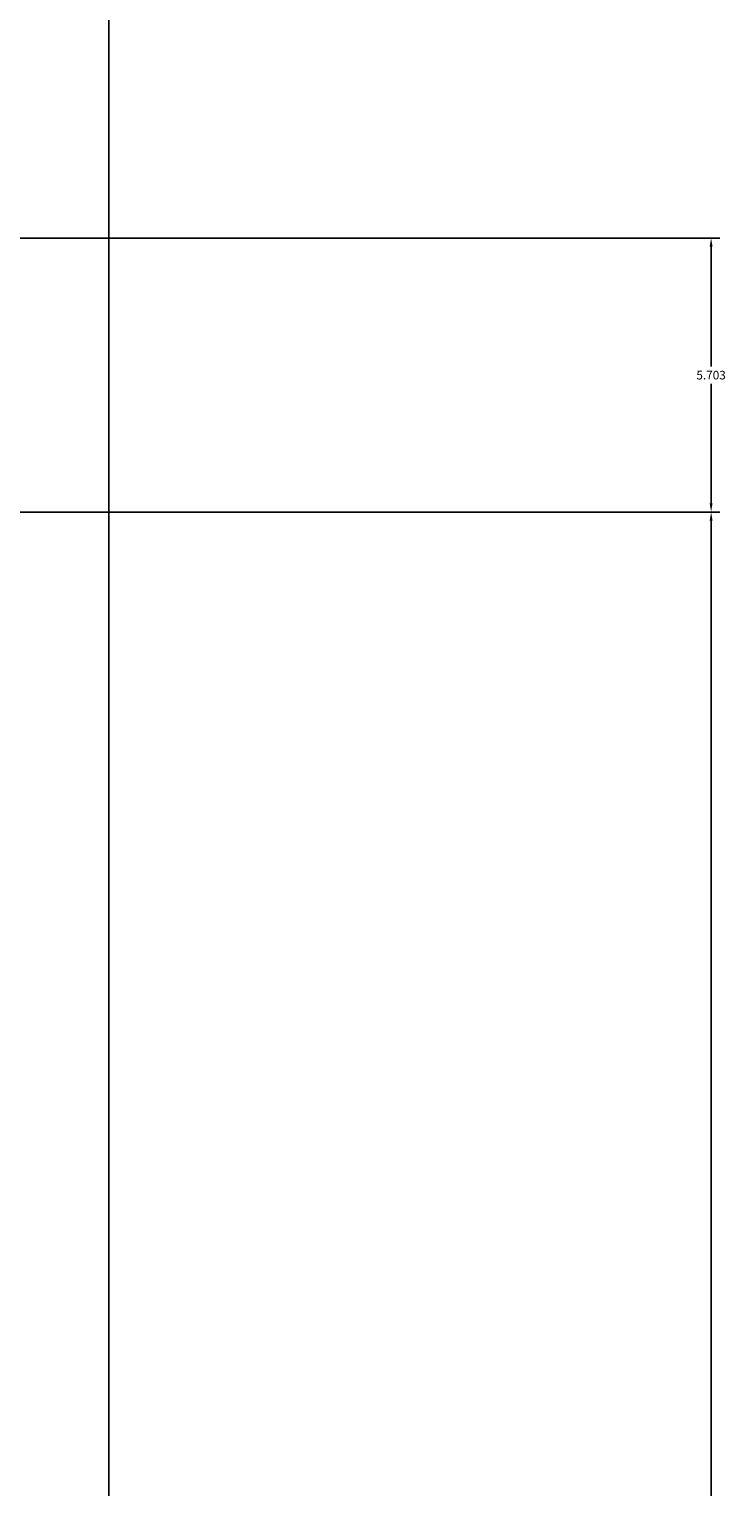
# Model space of a CAD drawing. Units: inches. Extents: x 2812 to 3051, y 1398 to 1659.
# Tile 42 of 65: x 3037 to 3051, y 1468 to 1498. Entities that reach past the tile are written whole.
import ezdxf

# ---------------------------------------------------------------- set-up
doc = ezdxf.new("R2010")
doc.units = ezdxf.units.IN
doc.layers.add('A-ANNO-DIMS', color=2, linetype='Continuous', lineweight=18)
doc.styles.get("Standard").update_dxf_attribs({"font": 'arial.ttf'})
doc.dimstyles.get("Standard").update_dxf_attribs({"dimtxt": 0.18, "dimasz": 0.18, "dimexe": 0.18, "dimexo": 0.0625, "dimgap": 0.09, "dimtad": 0, "dimtih": 1, "dimtoh": 1, "dimdec": 4, "dimzin": 0, "dimdsep": 46, "dimtxsty": 'Standard', "dimcen": 0.09, "dimadec": 0, "dimazin": 0, "dimtfac": 1, "dimtdec": 4, "dimtofl": 0, "dimtmove": 0, "dimatfit": 3, "dimfxl": 1, "dimtolj": 1, "dimtzin": 0, "dimarcsym": 0})

# ---------------------------------------------------------------- blocks, each defined once
blk = doc.blocks.new('*D34')
at = {"layer": 'A-ANNO-DIMS', "color": 0, "lineweight": -2, "transparency": 16777216}
for p, q in [((3038.462, 1593.482), (3038.462, 1397.505)), ((3027.385, 1550.757), (3027.385, 1397.505)), ((3027.565, 1397.685), (3032.468, 1397.685)), ((3038.282, 1397.685), (3033.379, 1397.685))]:
    blk.add_line(p, q, dxfattribs=at)
at = {"layer": 'A-ANNO-DIMS', "color": 0, "transparency": 16777216}
for points in [[(3027.565, 1397.715), (3027.565, 1397.655), (3027.385, 1397.685)], [(3038.282, 1397.715), (3038.282, 1397.655), (3038.462, 1397.685)]]:
    blk.add_solid(points, dxfattribs=at)
at = {"layer": 'Defpoints', "color": 0, "transparency": 16777216}
for p in [(3038.462, 1593.544), (3027.385, 1550.82), (3038.462, 1397.685)]:
    blk.add_point(p, dxfattribs=at)
at = {"layer": 'A-ANNO-DIMS', "color": 0, "transparency": 16777216, "insert": (3032.923, 1397.685), "char_height": 0.18, "attachment_point": 5}
blk.add_mtext('\\A1;11.077', dxfattribs=at)
blk = doc.blocks.new('*D54')
at = {"layer": 'A-ANNO-DIMS', "color": 0, "lineweight": -2, "transparency": 16777216}
for p, q in [((3036.447, 1488.035), (3051.178, 1488.035)), ((3050.998, 1487.855), (3050.998, 1449.217)), ((3050.998, 1410.215), (3050.998, 1448.853)), ((3036.447, 1410.035), (3051.178, 1410.035))]:
    blk.add_line(p, q, dxfattribs=at)
at = {"layer": 'A-ANNO-DIMS', "color": 0, "transparency": 16777216}
for points in [[(3050.968, 1487.855), (3051.028, 1487.855), (3050.998, 1488.035)], [(3050.968, 1410.215), (3051.028, 1410.215), (3050.998, 1410.035)]]:
    blk.add_solid(points, dxfattribs=at)
at = {"layer": 'Defpoints', "color": 0, "transparency": 16777216}
for p in [(3036.385, 1488.035), (3050.998, 1488.035), (3036.385, 1410.035)]:
    blk.add_point(p, dxfattribs=at)
at = {"layer": 'A-ANNO-DIMS', "color": 0, "transparency": 16777216, "insert": (3050.998, 1449.035), "char_height": 0.18, "attachment_point": 5}
blk.add_mtext('\\A1;78', dxfattribs=at)
blk = doc.blocks.new('*D55')
at = {"layer": 'A-ANNO-DIMS', "color": 0, "lineweight": -2, "transparency": 16777216}
for p, q in [((2850.811, 1493.738), (3051.178, 1493.738)), ((3050.998, 1493.558), (3050.998, 1491.069)), ((3050.998, 1488.215), (3050.998, 1490.705)), ((2850.811, 1488.035), (3051.178, 1488.035))]:
    blk.add_line(p, q, dxfattribs=at)
at = {"layer": 'A-ANNO-DIMS', "color": 0, "transparency": 16777216}
for points in [[(3050.968, 1493.558), (3051.028, 1493.558), (3050.998, 1493.738)], [(3050.968, 1488.215), (3051.028, 1488.215), (3050.998, 1488.035)]]:
    blk.add_solid(points, dxfattribs=at)
at = {"layer": 'Defpoints', "color": 0, "transparency": 16777216}
for p in [(2850.748, 1493.738), (3050.998, 1493.738), (2850.748, 1488.035)]:
    blk.add_point(p, dxfattribs=at)
at = {"layer": 'A-ANNO-DIMS', "color": 0, "transparency": 16777216, "insert": (3050.998, 1490.887), "char_height": 0.18, "attachment_point": 5}
blk.add_mtext('\\A1;5.703', dxfattribs=at)

msp = doc.modelspace()

# ---------------------------------------------------------------- dimensions: what is measured, and where the dimension line sits
at = {"layer": 'A-ANNO-DIMS'}
dim = msp.add_linear_dim(base=(3038.4621, 1397.6854), p1=(3027.3849, 1550.82), p2=(3038.4621, 1593.5441), dimstyle='Standard', override={"dimdec": 3, "dimlfac": 1, "dimrnd": 0, "dimzin": 0, "dimdsep": 46, "dimlunit": 2}, dxfattribs=at)
dim.commit()
dim.dimension.update_dxf_attribs({"geometry": '*D34', "text_midpoint": (3032.9235, 1397.6854)})
for base, p1, p2, override, picture, middle in [((3050.998, 1493.7383), (2850.7485, 1488.0354), (2850.7485, 1493.7383), {"dimdec": 3, "dimlfac": 1, "dimrnd": 0, "dimzin": 0, "dimdsep": 46, "dimlunit": 2}, '*D55', (3050.998, 1490.8868)), ((3050.998, 1488.0354), (3036.3849, 1410.0354), (3036.3849, 1488.0354), {"dimdec": 0, "dimlfac": 1, "dimrnd": 0, "dimzin": 0, "dimdsep": 46, "dimlunit": 2}, '*D54', (3050.998, 1449.0354))]:
    dim = msp.add_linear_dim(base=base, p1=p1, p2=p2, angle=90, dimstyle='Standard', override=override, dxfattribs=at)
    dim.commit()
    dim.dimension.update_dxf_attribs({"geometry": picture, "text_midpoint": middle})

doc.saveas('drawing.dxf')
